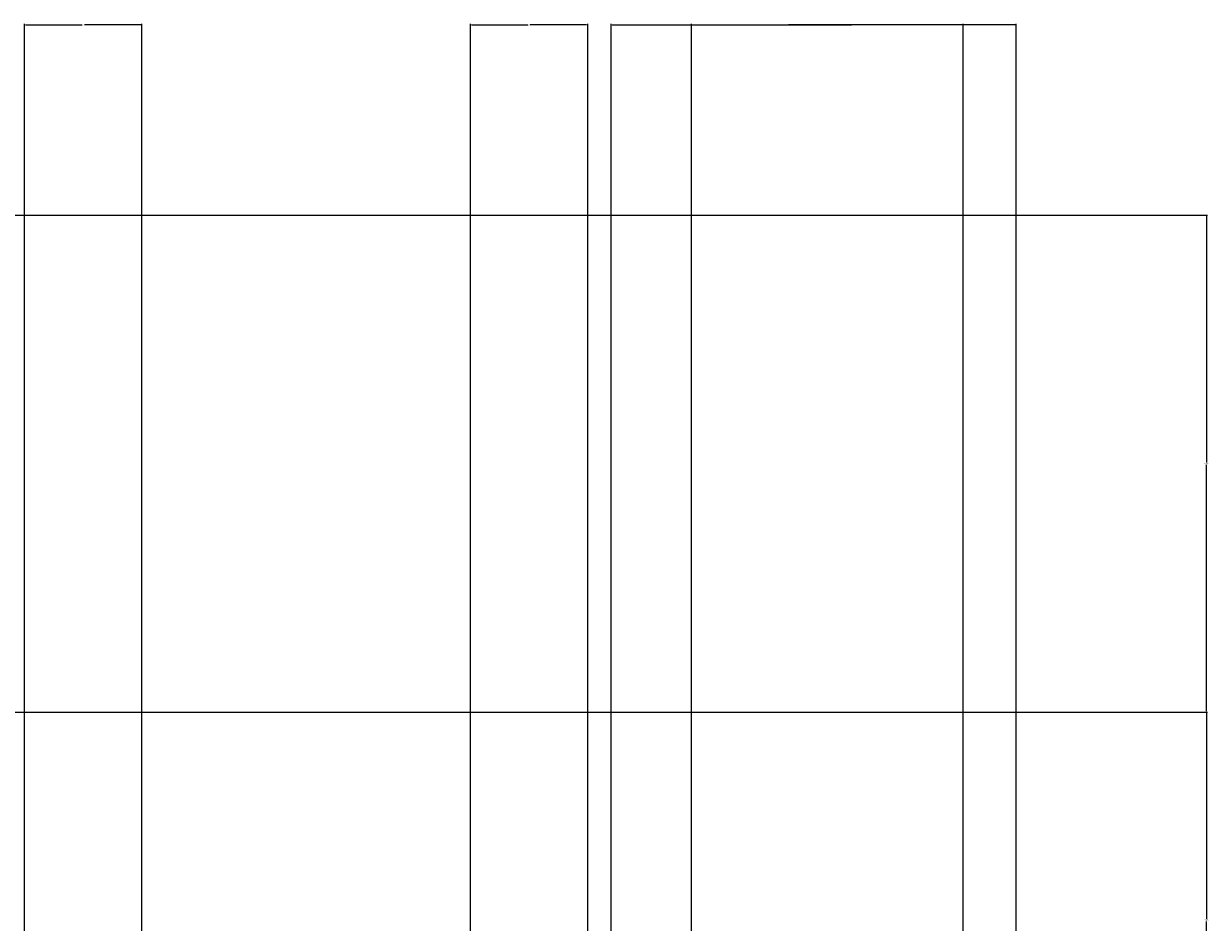
# Model space of a CAD drawing. Units: inches. Extents: x 821 to 2399, y 74 to 823.
# Tile 8 of 13: x 1128 to 1330, y 634 to 787. Entities that reach past the tile are written whole.
import ezdxf

# ---------------------------------------------------------------- set-up
doc = ezdxf.new("R2010")
doc.units = ezdxf.units.IN
doc.header["$MEASUREMENT"] = 0
doc.layers.add('A-ANNO-DIMS', color=2, linetype='Continuous', lineweight=18)
doc.styles.get("Standard").update_dxf_attribs({"font": 'arial.ttf'})
doc.dimstyles.get("Standard").update_dxf_attribs({"dimtxt": 0.18, "dimasz": 0.18, "dimexe": 0.18, "dimexo": 0.0625, "dimgap": 0.09, "dimtad": 0, "dimtih": 1, "dimtoh": 1, "dimdec": 4, "dimzin": 0, "dimdsep": 46, "dimtxsty": 'Standard', "dimcen": 0.09, "dimadec": 0, "dimazin": 0, "dimtfac": 1, "dimtdec": 4, "dimtofl": 0, "dimtmove": 0, "dimatfit": 3, "dimfxl": 1, "dimtolj": 1, "dimtzin": 0, "dimarcsym": 0})

# ---------------------------------------------------------------- blocks, each defined once
blk = doc.blocks.new('*D86')
at = {"layer": 'A-ANNO-DIMS', "color": 0, "lineweight": -2, "transparency": 16777216}
for p, q in [((1048.78, 754.12), (1330, 754.12)), ((1329.82, 753.94), (1329.82, 711.98)), ((1329.82, 669.65), (1329.82, 711.61)), ((1048.78, 669.47), (1330, 669.47))]:
    blk.add_line(p, q, dxfattribs=at)
at = {"layer": 'A-ANNO-DIMS', "color": 0, "lineweight": 50, "transparency": 16777216}
for points in [[(1329.79, 753.94), (1329.85, 753.94), (1329.82, 754.12)], [(1329.79, 669.65), (1329.85, 669.65), (1329.82, 669.47)]]:
    blk.add_solid(points, dxfattribs=at)
at = {"layer": 'Defpoints', "color": 0, "lineweight": 50, "transparency": 16777216}
for p in [(1048.72, 754.12), (1048.72, 669.47), (1329.82, 669.47)]:
    blk.add_point(p, dxfattribs=at)
at = {"layer": 'A-ANNO-DIMS', "color": 0, "transparency": 16777216, "insert": (1329.82, 711.79), "char_height": 0.18, "attachment_point": 5}
blk.add_mtext('\\A1;84.64', dxfattribs=at)
blk = doc.blocks.new('*D87')
at = {"layer": 'A-ANNO-DIMS', "color": 0, "lineweight": -2, "transparency": 16777216}
for p, q in [((1122.09, 669.47), (1330, 669.47)), ((1329.82, 669.29), (1329.82, 634.18)), ((1329.82, 598.7), (1329.82, 633.81)), ((1122.09, 598.52), (1330, 598.52))]:
    blk.add_line(p, q, dxfattribs=at)
at = {"layer": 'A-ANNO-DIMS', "color": 0, "lineweight": 50, "transparency": 16777216}
for points in [[(1329.79, 669.29), (1329.85, 669.29), (1329.82, 669.47)], [(1329.79, 598.7), (1329.85, 598.7), (1329.82, 598.52)]]:
    blk.add_solid(points, dxfattribs=at)
at = {"layer": 'Defpoints', "color": 0, "lineweight": 50, "transparency": 16777216}
for p in [(1122.03, 669.47), (1122.03, 598.52), (1329.82, 598.52)]:
    blk.add_point(p, dxfattribs=at)
at = {"layer": 'A-ANNO-DIMS', "color": 0, "transparency": 16777216, "insert": (1329.82, 634), "char_height": 0.18, "attachment_point": 5}
blk.add_mtext('\\A1;70.95', dxfattribs=at)
blk = doc.blocks.new('*D92')
at = {"layer": 'A-ANNO-DIMS', "color": 0, "lineweight": -2, "transparency": 16777216}
for p, q in [((1128.37, 209.58), (1128.37, 786.75)), ((1128.55, 786.57), (1138.15, 786.57)), ((1148.19, 786.57), (1138.59, 786.57)), ((1148.37, 209.58), (1148.37, 786.75))]:
    blk.add_line(p, q, dxfattribs=at)
at = {"layer": 'A-ANNO-DIMS', "color": 0, "lineweight": 50, "transparency": 16777216}
for points in [[(1128.55, 786.6), (1128.55, 786.54), (1128.37, 786.57)], [(1148.19, 786.6), (1148.19, 786.54), (1148.37, 786.57)]]:
    blk.add_solid(points, dxfattribs=at)
at = {"layer": 'Defpoints', "color": 0, "lineweight": 50, "transparency": 16777216}
for p in [(1148.37, 786.57), (1128.37, 209.52), (1148.37, 209.52)]:
    blk.add_point(p, dxfattribs=at)
at = {"layer": 'A-ANNO-DIMS', "color": 0, "transparency": 16777216, "insert": (1138.37, 786.57), "char_height": 0.18, "attachment_point": 5}
blk.add_mtext('\\A1;20', dxfattribs=at)
blk = doc.blocks.new('*D94')
at = {"layer": 'A-ANNO-DIMS', "color": 0, "lineweight": -2, "transparency": 16777216}
for p, q in [((1204.37, 396.58), (1204.37, 786.75)), ((1204.55, 786.57), (1214.15, 786.57)), ((1224.19, 786.57), (1214.59, 786.57)), ((1224.37, 396.58), (1224.37, 786.75))]:
    blk.add_line(p, q, dxfattribs=at)
at = {"layer": 'A-ANNO-DIMS', "color": 0, "lineweight": 50, "transparency": 16777216}
for points in [[(1204.55, 786.6), (1204.55, 786.54), (1204.37, 786.57)], [(1224.19, 786.6), (1224.19, 786.54), (1224.37, 786.57)]]:
    blk.add_solid(points, dxfattribs=at)
at = {"layer": 'Defpoints', "color": 0, "lineweight": 50, "transparency": 16777216}
for p in [(1224.37, 786.57), (1204.37, 396.52), (1224.37, 396.52)]:
    blk.add_point(p, dxfattribs=at)
at = {"layer": 'A-ANNO-DIMS', "color": 0, "transparency": 16777216, "insert": (1214.37, 786.57), "char_height": 0.18, "attachment_point": 5}
blk.add_mtext('\\A1;20', dxfattribs=at)
blk = doc.blocks.new('*D95')
at = {"layer": 'A-ANNO-DIMS', "color": 0, "lineweight": -2, "transparency": 16777216}
for p, q in [((1228.37, 396.58), (1228.37, 786.75)), ((1228.55, 786.57), (1258.15, 786.57)), ((1288.19, 786.57), (1258.59, 786.57)), ((1288.37, 396.58), (1288.37, 786.75))]:
    blk.add_line(p, q, dxfattribs=at)
at = {"layer": 'A-ANNO-DIMS', "color": 0, "lineweight": 50, "transparency": 16777216}
for points in [[(1228.55, 786.6), (1228.55, 786.54), (1228.37, 786.57)], [(1288.19, 786.6), (1288.19, 786.54), (1288.37, 786.57)]]:
    blk.add_solid(points, dxfattribs=at)
at = {"layer": 'Defpoints', "color": 0, "lineweight": 50, "transparency": 16777216}
for p in [(1288.37, 786.57), (1228.37, 396.52), (1288.37, 396.52)]:
    blk.add_point(p, dxfattribs=at)
at = {"layer": 'A-ANNO-DIMS', "color": 0, "transparency": 16777216, "insert": (1258.37, 786.57), "char_height": 0.18, "attachment_point": 5}
blk.add_mtext('\\A1;60', dxfattribs=at)
blk = doc.blocks.new('*D98')
at = {"layer": 'A-ANNO-DIMS', "color": 0, "lineweight": -2, "transparency": 16777216}
for p, q in [((1242.03, 597.58), (1242.03, 786.75)), ((1242.21, 786.57), (1269.31, 786.57)), ((1297.19, 786.57), (1270.09, 786.57)), ((1297.37, 598.58), (1297.37, 786.75))]:
    blk.add_line(p, q, dxfattribs=at)
at = {"layer": 'A-ANNO-DIMS', "color": 0, "lineweight": 50, "transparency": 16777216}
for points in [[(1242.21, 786.6), (1242.21, 786.54), (1242.03, 786.57)], [(1297.19, 786.6), (1297.19, 786.54), (1297.37, 786.57)]]:
    blk.add_solid(points, dxfattribs=at)
at = {"layer": 'Defpoints', "color": 0, "lineweight": 50, "transparency": 16777216}
for p in [(1297.37, 786.57), (1297.37, 598.52), (1242.03, 597.52)]:
    blk.add_point(p, dxfattribs=at)
at = {"layer": 'A-ANNO-DIMS', "color": 0, "transparency": 16777216, "insert": (1269.7, 786.57), "char_height": 0.18, "attachment_point": 5}
blk.add_mtext('\\A1;55.35', dxfattribs=at)

msp = doc.modelspace()

# ---------------------------------------------------------------- dimensions: what is measured, and where the dimension line sits
at = {"layer": 'A-ANNO-DIMS'}
for base, p1, p2, override, picture, middle in [((1148.3735, 786.5664), (1128.3735, 209.5195), (1148.3735, 209.5195), {"dimdec": 0, "dimlfac": 1, "dimrnd": 0, "dimzin": 0, "dimdsep": 46, "dimlunit": 2}, '*D92', (1138.3735, 786.5664)), ((1224.3735, 786.5664), (1204.3735, 396.5195), (1224.3735, 396.5195), {"dimdec": 0, "dimlfac": 1, "dimrnd": 0, "dimzin": 0, "dimdsep": 46, "dimlunit": 2}, '*D94', (1214.3735, 786.5664)), ((1288.3735, 786.5664), (1228.3735, 396.5195), (1288.3735, 396.5195), {"dimdec": 0, "dimlfac": 1, "dimrnd": 0, "dimzin": 0, "dimdsep": 46, "dimlunit": 2}, '*D95', (1258.3735, 786.5664)), ((1297.3735, 786.5664), (1242.0276, 597.5195), (1297.3735, 598.5195), {"dimdec": 2, "dimlfac": 1, "dimrnd": 0, "dimzin": 0, "dimdsep": 46, "dimlunit": 2}, '*D98', (1269.7005, 786.5664))]:
    dim = msp.add_linear_dim(base=base, p1=p1, p2=p2, dimstyle='Standard', override=override, dxfattribs=at)
    dim.commit()
    dim.dimension.update_dxf_attribs({"geometry": picture, "text_midpoint": middle})
for base, p1, p2, picture, middle in [((1329.8235, 669.4726), (1048.7194, 754.1164), (1048.7194, 669.4726), '*D86', (1329.8235, 711.7945)), ((1329.8235, 598.5195), (1122.0283, 669.4726), (1122.0283, 598.5195), '*D87', (1329.8235, 633.996))]:
    dim = msp.add_linear_dim(base=base, p1=p1, p2=p2, angle=90, dimstyle='Standard', override={"dimdec": 2, "dimlfac": 1, "dimrnd": 0, "dimzin": 0, "dimdsep": 46, "dimlunit": 2}, dxfattribs=at)
    dim.commit()
    dim.dimension.update_dxf_attribs({"geometry": picture, "text_midpoint": middle})

doc.saveas('drawing.dxf')
